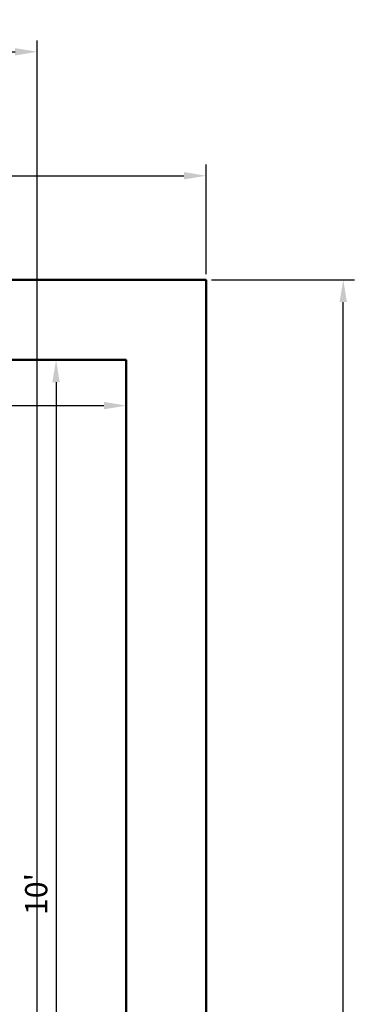
# Model space of a CAD drawing. Units: inches. Extents: x 2385 to 2740, y 1752 to 2305.
# Tile 15 of 15: x 2691 to 2729, y 2195 to 2305. Entities that reach past the tile are written whole.
import ezdxf

# ---------------------------------------------------------------- set-up
doc = ezdxf.new("R2010")
doc.units = ezdxf.units.IN
doc.layers.add('A-ANNO-DIMS', color=2, linetype='Continuous', lineweight=18)
doc.layers.add('A-WALL', color=7, linetype='Continuous', lineweight=50)
doc.styles.get("Standard").update_dxf_attribs({"font": 'arial.ttf'})
doc.dimstyles.new('Copy of ISO-25', dxfattribs={"dimtxt": 2.5, "dimasz": 2.5, "dimexe": 1.25, "dimexo": 0.625, "dimtad": 1, "dimdec": 1, "dimlunit": 4, "dimtxsty": 'Standard', "dimcen": 2.5, "dimadec": 0, "dimazin": 0, "dimtfac": 1, "dimtdec": 1, "dimtmove": 0, "dimatfit": 3, "dimfxl": 1, "dimarcsym": 0})

# ---------------------------------------------------------------- blocks, each defined once
blk = doc.blocks.new('*D8')
at = {"layer": 'A-ANNO-DIMS', "color": 0, "lineweight": -2, "transparency": 16777216}
for p, q in [((2583.25, 2266.34), (2583.25, 2260.59)), ((2703.25, 2266.34), (2703.25, 2260.59)), ((2585.75, 2261.84), (2700.75, 2261.84))]:
    blk.add_line(p, q, dxfattribs=at)
at = {"layer": 'A-ANNO-DIMS', "color": 0, "transparency": 16777216}
for points in [[(2585.75, 2262.26), (2585.75, 2261.42), (2583.25, 2261.84)], [(2700.75, 2262.26), (2700.75, 2261.42), (2703.25, 2261.84)]]:
    blk.add_solid(points, dxfattribs=at)
at = {"layer": 'Defpoints', "color": 0, "transparency": 16777216}
for p in [(2583.25, 2266.97), (2703.25, 2266.97), (2703.25, 2261.84)]:
    blk.add_point(p, dxfattribs=at)
at = {"layer": 'A-ANNO-DIMS', "color": 0, "transparency": 16777216, "insert": (2643.25, 2263.74), "char_height": 2.5, "attachment_point": 5}
blk.add_mtext("10'", dxfattribs=at)
blk = doc.blocks.new('*D9')
at = {"layer": 'A-ANNO-DIMS', "color": 0, "lineweight": -2, "transparency": 16777216}
for p, q in [((2702.62, 2266.97), (2694.11, 2266.97)), ((2695.36, 2264.47), (2695.36, 2149.47)), ((2702.62, 2146.97), (2694.11, 2146.97))]:
    blk.add_line(p, q, dxfattribs=at)
at = {"layer": 'A-ANNO-DIMS', "color": 0, "transparency": 16777216}
for points in [[(2694.94, 2264.47), (2695.77, 2264.47), (2695.36, 2266.97)], [(2694.94, 2149.47), (2695.77, 2149.47), (2695.36, 2146.97)]]:
    blk.add_solid(points, dxfattribs=at)
at = {"layer": 'Defpoints', "color": 0, "transparency": 16777216}
for p in [(2703.25, 2266.97), (2695.36, 2146.97), (2703.25, 2146.97)]:
    blk.add_point(p, dxfattribs=at)
at = {"layer": 'A-ANNO-DIMS', "color": 0, "transparency": 16777216, "insert": (2693.45, 2206.97), "char_height": 2.5, "attachment_point": 5, "rotation": 90}
blk.add_mtext("10'", dxfattribs=at)
blk = doc.blocks.new('*D24')
at = {"layer": 'A-ANNO-DIMS', "color": 0, "lineweight": -2, "transparency": 16777216}
for p, q in [((2414.25, 2276.59), (2414.25, 2288.91)), ((2712.25, 2276.59), (2712.25, 2288.91)), ((2416.75, 2287.66), (2709.75, 2287.66))]:
    blk.add_line(p, q, dxfattribs=at)
at = {"layer": 'A-ANNO-DIMS', "color": 0, "transparency": 16777216}
for points in [[(2416.75, 2288.08), (2416.75, 2287.25), (2414.25, 2287.66)], [(2709.75, 2288.08), (2709.75, 2287.25), (2712.25, 2287.66)]]:
    blk.add_solid(points, dxfattribs=at)
at = {"layer": 'Defpoints', "color": 0, "transparency": 16777216}
for p in [(2712.25, 2287.66), (2414.25, 2275.97), (2712.25, 2275.97)]:
    blk.add_point(p, dxfattribs=at)
at = {"layer": 'A-ANNO-DIMS', "color": 0, "transparency": 16777216, "insert": (2563.25, 2289.57), "char_height": 2.5, "attachment_point": 5}
blk.add_mtext('24\'-10"', dxfattribs=at)
blk = doc.blocks.new('*D25')
at = {"layer": 'A-ANNO-DIMS', "color": 0, "lineweight": -2, "transparency": 16777216}
for p, q in [((2712.87, 2275.97), (2728.93, 2275.97)), ((2727.68, 1781.47), (2727.68, 2273.47)), ((2712.87, 1778.97), (2728.93, 1778.97))]:
    blk.add_line(p, q, dxfattribs=at)
at = {"layer": 'A-ANNO-DIMS', "color": 0, "transparency": 16777216}
for points in [[(2727.26, 2273.47), (2728.09, 2273.47), (2727.68, 2275.97)], [(2727.26, 1781.47), (2728.09, 1781.47), (2727.68, 1778.97)]]:
    blk.add_solid(points, dxfattribs=at)
at = {"layer": 'Defpoints', "color": 0, "transparency": 16777216}
for p in [(2712.25, 2275.97), (2727.68, 2275.97), (2712.25, 1778.97)]:
    blk.add_point(p, dxfattribs=at)
at = {"layer": 'A-ANNO-DIMS', "color": 0, "transparency": 16777216, "insert": (2725.77, 2027.47), "char_height": 2.5, "attachment_point": 5, "rotation": 90}
blk.add_mtext('41\'-5"', dxfattribs=at)
blk = doc.blocks.new('*D43')
at = {"layer": 'A-ANNO-DIMS', "color": 0, "lineweight": -2, "transparency": 16777216}
for p, q in [((2657.25, 1863.59), (2657.25, 2302.84)), ((2693.25, 1863.59), (2693.25, 2302.84)), ((2659.75, 2301.59), (2690.75, 2301.59))]:
    blk.add_line(p, q, dxfattribs=at)
at = {"layer": 'A-ANNO-DIMS', "color": 0, "transparency": 16777216}
for points in [[(2659.75, 2302), (2659.75, 2301.17), (2657.25, 2301.59)], [(2690.75, 2302), (2690.75, 2301.17), (2693.25, 2301.59)]]:
    blk.add_solid(points, dxfattribs=at)
at = {"layer": 'Defpoints', "color": 0, "transparency": 16777216}
for p in [(2693.25, 2301.59), (2657.25, 1862.97), (2693.25, 1862.97)]:
    blk.add_point(p, dxfattribs=at)
at = {"layer": 'A-ANNO-DIMS', "color": 0, "transparency": 16777216, "insert": (2675.25, 2303.49), "char_height": 2.5, "attachment_point": 5}
blk.add_mtext('3\'-0"', dxfattribs=at)

msp = doc.modelspace()

# ---------------------------------------------------------------- linework, layer by layer
at = {"layer": 'A-WALL'}
for p, q in [((2414.25, 2275.97), (2694.25, 2275.97)), ((2414.25, 2275.97), (2712.25, 2275.97)), ((2694.25, 2275.97), (2703.25, 2275.97)), ((2703.25, 2275.97), (2712.25, 2275.97)), ((2712.25, 2275.97), (2712.25, 2134.97)), ((2712.25, 2275.97), (2712.25, 2266.97)), ((2712.25, 2275.97), (2712.25, 1778.97)), ((2703.25, 2266.97), (2583.25, 2266.97)), ((2703.25, 2266.97), (2703.25, 2146.97))]:
    msp.add_line(p, q, dxfattribs=at)

# ---------------------------------------------------------------- dimensions: what is measured, and where the dimension line sits
at = {"layer": 'A-ANNO-DIMS'}
for base, p1, p2, override, picture, middle in [((2693.25, 2301.59), (2657.25, 1862.97), (2693.25, 1862.97), {"dimdec": 1, "dimlfac": 1, "dimrnd": 0, "dimzin": 1, "dimdsep": 46, "dimlunit": 4, "dimfrac": 2}, '*D43', (2675.25, 2303.49)), ((2712.25, 2287.66), (2414.25, 2275.97), (2712.25, 2275.97), {"dimclrd": 0, "dimclre": 0, "dimclrt": 0}, '*D24', (2563.25, 2289.57)), ((2703.25, 2261.84), (2583.25, 2266.97), (2703.25, 2266.97), {"dimclrd": 0, "dimclre": 0, "dimclrt": 0}, '*D8', (2643.25, 2263.74))]:
    dim = msp.add_linear_dim(base=base, p1=p1, p2=p2, dimstyle='Copy of ISO-25', override=override, dxfattribs=at)
    dim.commit()
    dim.dimension.update_dxf_attribs({"geometry": picture, "text_midpoint": middle})
for base, p1, p2, picture, middle in [((2727.68, 2275.97), (2712.25, 1778.97), (2712.25, 2275.97), '*D25', (2725.77, 2027.47)), ((2695.36, 2146.97), (2703.25, 2266.97), (2703.25, 2146.97), '*D9', (2693.45, 2206.97))]:
    dim = msp.add_linear_dim(base=base, p1=p1, p2=p2, angle=90, dimstyle='Copy of ISO-25', override={"dimclrd": 0, "dimclre": 0, "dimclrt": 0}, dxfattribs=at)
    dim.commit()
    dim.dimension.update_dxf_attribs({"geometry": picture, "text_midpoint": middle})

doc.saveas('drawing.dxf')
